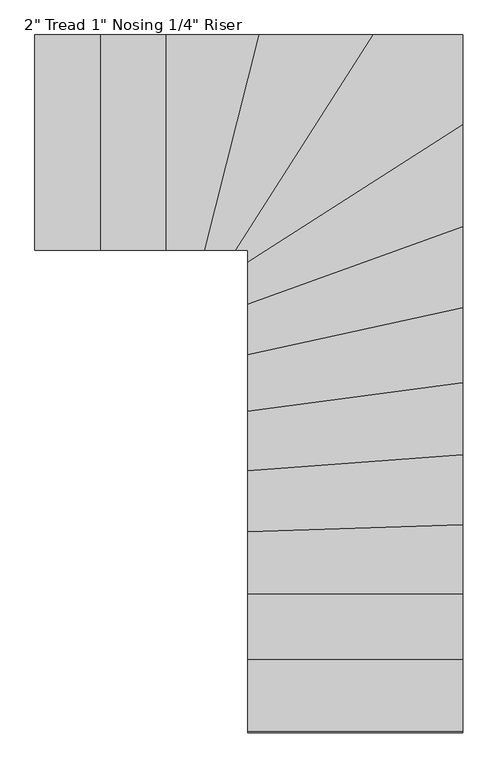
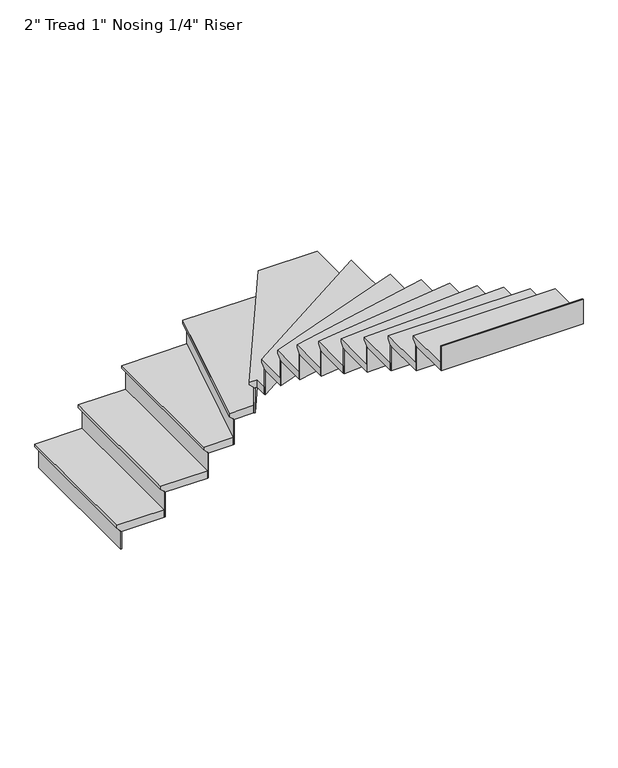
"""IFC4 building model written with IfcOpenShell, lengths in millimetres: stair flight geometry."""

from ifc_helpers import new_model, si_unit, origin, place, context, project, spatial, faceted_brep, source, transform, mapped, element, save


def stair_flight_29561c67(model_context):
    return source(origin(), model_context, "Body", "Brep", [
        faceted_brep([(-4406.7350785, 4803.7033005, 827.6166667), (-4406.7350785, 4803.7033005, 846.6666667), (-4406.7350785, 5718.1033005, 846.6666667), (-4406.7350785, 5718.1033005, 827.6166667), (-4381.3350785, 4803.7033005, 802.2166667), (-4381.3350785, 5718.1033005, 802.2166667), (-4101.9350785, 4803.7033005, 846.6666667), (-4101.9350785, 5718.1033005, 846.6666667), (-4381.3350785, 5718.1033005, 795.8666667), (-4101.9350785, 5718.1033005, 795.8666667), (-4101.9350785, 4803.7033005, 795.8666667), (-4381.3350785, 4803.7033005, 795.8666667)], [[[0, 1, 2, 3]], [[4, 0, 3, 5]], [[2, 1, 6, 7]], [[8, 9, 10, 11]], [[2, 7, 9, 8, 5, 3]], [[8, 11, 4, 5]], [[6, 1, 0, 4, 11, 10]], [[7, 6, 10, 9]]]),
        faceted_brep([(-4381.3350785, 4803.7033005, 795.8666667), (-4381.3350785, 4803.7033005, 677.3333333), (-4374.9850785, 4803.7033005, 677.3333333), (-4374.9850785, 4803.7033005, 795.8666667), (-4381.3350785, 5718.1033005, 795.8666667), (-4374.9850785, 5718.1033005, 795.8666667), (-4374.9850785, 5718.1033005, 677.3333333), (-4381.3350785, 5718.1033005, 677.3333333)], [[[0, 1, 2, 3]], [[4, 5, 6, 7]], [[1, 0, 4, 7]], [[2, 1, 7, 6]], [[3, 2, 6, 5]], [[0, 3, 5, 4]]]),
        faceted_brep([(-4101.9350785, 4803.7033005, 965.2), (-4101.9350785, 4803.7033005, 795.8666667), (-4095.5850785, 4803.7033005, 795.8666667), (-4095.5850785, 4803.7033005, 965.2), (-4101.9350785, 5718.1033005, 965.2), (-4095.5850785, 5718.1033005, 965.2), (-4095.5850785, 5718.1033005, 795.8666667), (-4101.9350785, 5718.1033005, 795.8666667)], [[[0, 1, 2, 3]], [[4, 5, 6, 7]], [[1, 0, 4, 7]], [[2, 1, 7, 6]], [[3, 2, 6, 5]], [[0, 3, 5, 4]]]),
        faceted_brep([(-4127.3350785, 5718.1033005, 1016.0), (-4127.3350785, 4803.7033005, 1016.0), (-3822.5350785, 4803.7033005, 1016.0), (-3822.5350785, 5718.1033005, 1016.0), (-4101.9350785, 5718.1033005, 965.2), (-3822.5350785, 5718.1033005, 965.2), (-3822.5350785, 4803.7033005, 965.2), (-4101.9350785, 4803.7033005, 965.2), (-4101.9350785, 5718.1033005, 971.55), (-4127.3350785, 5718.1033005, 996.95), (-4101.9350785, 4803.7033005, 971.55), (-4127.3350785, 4803.7033005, 996.95)], [[[0, 1, 2, 3]], [[4, 5, 6, 7]], [[0, 3, 5, 4, 8, 9]], [[4, 7, 10, 8]], [[2, 1, 11, 10, 7, 6]], [[3, 2, 6, 5]], [[11, 1, 0, 9]], [[10, 11, 9, 8]]]),
        faceted_brep([(-3822.5350785, 4803.7033005, 1134.5333333), (-3822.5350785, 4803.7033005, 965.2), (-3816.1850785, 4803.7033005, 965.2), (-3816.1850785, 4803.7033005, 1134.5333333), (-3822.5350785, 5718.1033005, 1134.5333333), (-3816.1850785, 5718.1033005, 1134.5333333), (-3816.1850785, 5718.1033005, 965.2), (-3822.5350785, 5718.1033005, 965.2)], [[[0, 1, 2, 3]], [[4, 5, 6, 7]], [[1, 0, 4, 7]], [[2, 1, 7, 6]], [[3, 2, 6, 5]], [[0, 3, 5, 4]]]),
        faceted_brep([(-3847.9350785, 5718.1033005, 1185.3333333), (-3847.9350785, 4803.7033005, 1185.3333333), (-3657.8300447, 4803.7033005, 1185.3333333), (-3426.8443681, 5718.1033005, 1185.3333333), (-3822.5350785, 5718.1033005, 1134.5333333), (-3426.8443681, 5718.1033005, 1134.5333333), (-3657.8300447, 4803.7033005, 1134.5333333), (-3822.5350785, 4803.7033005, 1134.5333333), (-3822.5350785, 5718.1033005, 1140.8833333), (-3847.9350785, 5718.1033005, 1166.2833333), (-3822.5350785, 4803.7033005, 1140.8833333), (-3847.9350785, 4803.7033005, 1166.2833333)], [[[0, 1, 2, 3]], [[4, 5, 6, 7]], [[0, 3, 5, 4, 8, 9]], [[4, 7, 10, 8]], [[2, 1, 11, 10, 7, 6]], [[3, 2, 6, 5]], [[11, 1, 0, 9]], [[10, 11, 9, 8]]]),
        faceted_brep([(-3657.8300447, 4803.7033005, 1303.8666667), (-3657.8300447, 4803.7033005, 1134.5333333), (-3651.2805766, 4803.7033005, 1134.5333333), (-3651.2805766, 4803.7033005, 1303.8666667), (-3426.8443681, 5718.1033005, 1303.8666667), (-3420.2949, 5718.1033005, 1303.8666667), (-3420.2949, 5718.1033005, 1134.5333333), (-3426.8443681, 5718.1033005, 1134.5333333)], [[[0, 1, 2, 3]], [[4, 5, 6, 7]], [[1, 0, 4, 7]], [[2, 1, 7, 6]], [[3, 2, 6, 5]], [[0, 3, 5, 4]]]),
        faceted_brep([(-3453.0422402, 5718.1033005, 1354.6666667), (-3684.0279168, 4803.7033005, 1354.6666667), (-3523.5624556, 4803.7033005, 1354.6666667), (-2938.9630202, 5718.1033005, 1354.6666667), (-3426.8443681, 5718.1033005, 1303.8666667), (-2938.9630202, 5718.1033005, 1303.8666667), (-3523.5624556, 4803.7033005, 1303.8666667), (-3657.8300447, 4803.7033005, 1303.8666667), (-3426.8443681, 5718.1033005, 1310.2166667), (-3453.0422402, 5718.1033005, 1335.6166667), (-3657.8300447, 4803.7033005, 1310.2166667), (-3684.0279168, 4803.7033005, 1335.6166667)], [[[0, 1, 2, 3]], [[4, 5, 6, 7]], [[0, 3, 5, 4, 8, 9]], [[4, 7, 10, 8]], [[2, 1, 11, 10, 7, 6]], [[3, 2, 6, 5]], [[11, 1, 0, 9]], [[10, 11, 9, 8]]]),
        faceted_brep([(-3523.5624556, 4803.7033005, 1473.2), (-3523.5624556, 4803.7033005, 1303.8666667), (-3516.0256252, 4803.7033005, 1303.8666667), (-3516.0256252, 4803.7033005, 1473.2), (-2938.9630202, 5718.1033005, 1473.2), (-2931.4261898, 5718.1033005, 1473.2), (-2931.4261898, 5718.1033005, 1303.8666667), (-2938.9630202, 5718.1033005, 1303.8666667)], [[[0, 1, 2, 3]], [[4, 5, 6, 7]], [[1, 0, 4, 7]], [[2, 1, 7, 6]], [[3, 2, 6, 5]], [[0, 3, 5, 4]]]),
        faceted_brep([(-2588.398089, 5307.243726, 1524.0), (-2588.398089, 5718.1033005, 1524.0), (-2969.1103419, 5718.1033005, 1524.0), (-3553.7097773, 4803.7033005, 1524.0), (-3502.798089, 4803.7033005, 1524.0), (-3502.798089, 4722.6442906, 1524.0), (-2588.398089, 5718.1033005, 1473.2), (-2588.398089, 5307.243726, 1473.2), (-3502.798089, 4722.6442906, 1473.2), (-3502.798089, 4803.7033005, 1473.2), (-3523.5624556, 4803.7033005, 1473.2), (-2938.9630202, 5718.1033005, 1473.2), (-3523.5624556, 4803.7033005, 1479.55), (-2938.9630202, 5718.1033005, 1479.55), (-3553.7097773, 4803.7033005, 1504.95), (-2969.1103419, 5718.1033005, 1504.95)], [[[0, 1, 2, 3, 4, 5]], [[6, 7, 8, 9, 10, 11]], [[1, 0, 7, 6]], [[11, 10, 12, 13]], [[4, 3, 14, 12, 10, 9]], [[0, 5, 8, 7]], [[14, 3, 2, 15]], [[12, 14, 15, 13]], [[2, 1, 6, 11, 13, 15]], [[5, 4, 9, 8]]]),
        faceted_brep([(-3502.798089, 4722.6442906, 1642.5333333), (-3502.798089, 4722.6442906, 1473.2), (-3502.798089, 4715.1074602, 1473.2), (-3502.798089, 4715.1074602, 1642.5333333), (-2588.398089, 5307.243726, 1642.5333333), (-2588.398089, 5299.7068956, 1642.5333333), (-2588.398089, 5299.7068956, 1473.2), (-2588.398089, 5307.243726, 1473.2)], [[[0, 1, 2, 3]], [[4, 5, 6, 7]], [[1, 0, 4, 7]], [[2, 1, 7, 6]], [[3, 2, 6, 5]], [[0, 3, 5, 4]]]),
        faceted_brep([(-2588.398089, 5337.3910477, 1693.3333333), (-3502.798089, 4752.7916123, 1693.3333333), (-3502.798089, 4546.6879787, 1693.3333333), (-2588.398089, 4875.2644835, 1693.3333333), (-2588.398089, 5307.243726, 1642.5333333), (-2588.398089, 4875.2644835, 1642.5333333), (-3502.798089, 4546.6879787, 1642.5333333), (-3502.798089, 4722.6442906, 1642.5333333), (-2588.398089, 5307.243726, 1648.8833333), (-2588.398089, 5337.3910477, 1674.2833333), (-3502.798089, 4722.6442906, 1648.8833333), (-3502.798089, 4752.7916123, 1674.2833333)], [[[0, 1, 2, 3]], [[4, 5, 6, 7]], [[0, 3, 5, 4, 8, 9]], [[4, 7, 10, 8]], [[2, 1, 11, 10, 7, 6]], [[3, 2, 6, 5]], [[11, 1, 0, 9]], [[10, 11, 9, 8]]]),
        faceted_brep([(-3502.798089, 4546.6879787, 1811.8666667), (-3502.798089, 4546.6879787, 1642.5333333), (-3502.798089, 4539.9404588, 1642.5333333), (-3502.798089, 4539.9404588, 1811.8666667), (-2588.398089, 4875.2644835, 1811.8666667), (-2588.398089, 4868.5169635, 1811.8666667), (-2588.398089, 4868.5169635, 1642.5333333), (-2588.398089, 4875.2644835, 1642.5333333)], [[[0, 1, 2, 3]], [[4, 5, 6, 7]], [[1, 0, 4, 7]], [[2, 1, 7, 6]], [[3, 2, 6, 5]], [[0, 3, 5, 4]]]),
        faceted_brep([(-2588.398089, 4902.2545634, 1862.6666667), (-3502.798089, 4573.6780586, 1862.6666667), (-3502.798089, 4332.5715797, 1862.6666667), (-2588.398089, 4532.5602463, 1862.6666667), (-2588.398089, 4875.2644835, 1811.8666667), (-2588.398089, 4532.5602463, 1811.8666667), (-3502.798089, 4332.5715797, 1811.8666667), (-3502.798089, 4546.6879787, 1811.8666667), (-2588.398089, 4875.2644835, 1818.2166667), (-2588.398089, 4902.2545634, 1843.6166667), (-3502.798089, 4546.6879787, 1818.2166667), (-3502.798089, 4573.6780586, 1843.6166667)], [[[0, 1, 2, 3]], [[4, 5, 6, 7]], [[0, 3, 5, 4, 8, 9]], [[4, 7, 10, 8]], [[2, 1, 11, 10, 7, 6]], [[3, 2, 6, 5]], [[11, 1, 0, 9]], [[10, 11, 9, 8]]]),
        faceted_brep([(-3502.798089, 4332.5715797, 1981.2), (-3502.798089, 4332.5715797, 1811.8666667), (-3502.798089, 4326.0714802, 1811.8666667), (-3502.798089, 4326.0714802, 1981.2), (-2588.398089, 4532.5602463, 1981.2), (-2588.398089, 4526.0601468, 1981.2), (-2588.398089, 4526.0601468, 1811.8666667), (-2588.398089, 4532.5602463, 1811.8666667)], [[[0, 1, 2, 3]], [[4, 5, 6, 7]], [[1, 0, 4, 7]], [[2, 1, 7, 6]], [[3, 2, 6, 5]], [[0, 3, 5, 4]]]),
        faceted_brep([(-2588.398089, 4558.5606443, 2032.0), (-3502.798089, 4358.5719777, 2032.0), (-3502.798089, 4093.0245396, 2032.0), (-2588.398089, 4214.0649516, 2032.0), (-2588.398089, 4532.5602463, 1981.2), (-2588.398089, 4214.0649516, 1981.2), (-3502.798089, 4093.0245396, 1981.2), (-3502.798089, 4332.5715797, 1981.2), (-2588.398089, 4532.5602463, 1987.55), (-2588.398089, 4558.5606443, 2012.95), (-3502.798089, 4332.5715797, 1987.55), (-3502.798089, 4358.5719777, 2012.95)], [[[0, 1, 2, 3]], [[4, 5, 6, 7]], [[0, 3, 5, 4, 8, 9]], [[4, 7, 10, 8]], [[2, 1, 11, 10, 7, 6]], [[3, 2, 6, 5]], [[11, 1, 0, 9]], [[10, 11, 9, 8]]]),
        faceted_brep([(-3502.798089, 4093.0245396, 2150.5333333), (-3502.798089, 4093.0245396, 1981.2), (-3502.798089, 4086.6191482, 1981.2), (-3502.798089, 4086.6191482, 2150.5333333), (-2588.398089, 4214.0649516, 2150.5333333), (-2588.398089, 4207.6595603, 2150.5333333), (-2588.398089, 4207.6595603, 1981.2), (-2588.398089, 4214.0649516, 1981.2)], [[[0, 1, 2, 3]], [[4, 5, 6, 7]], [[1, 0, 4, 7]], [[2, 1, 7, 6]], [[3, 2, 6, 5]], [[0, 3, 5, 4]]]),
        faceted_brep([(-2588.398089, 4239.6865171, 2201.3333333), (-3502.798089, 4118.646105, 2201.3333333), (-3502.798089, 3840.4778148, 2201.3333333), (-2588.398089, 3908.1160191, 2201.3333333), (-2588.398089, 4214.0649516, 2150.5333333), (-2588.398089, 3908.1160191, 2150.5333333), (-3502.798089, 3840.4778148, 2150.5333333), (-3502.798089, 4093.0245396, 2150.5333333), (-2588.398089, 4214.0649516, 2156.8833333), (-2588.398089, 4239.6865171, 2182.2833333), (-3502.798089, 4093.0245396, 2156.8833333), (-3502.798089, 4118.646105, 2182.2833333)], [[[0, 1, 2, 3]], [[4, 5, 6, 7]], [[0, 3, 5, 4, 8, 9]], [[4, 7, 10, 8]], [[2, 1, 11, 10, 7, 6]], [[3, 2, 6, 5]], [[11, 1, 0, 9]], [[10, 11, 9, 8]]]),
        faceted_brep([(-3502.798089, 3840.4778148, 2319.8666667), (-3502.798089, 3840.4778148, 2150.5333333), (-3502.798089, 3834.1104663, 2150.5333333), (-3502.798089, 3834.1104663, 2319.8666667), (-2588.398089, 3908.1160191, 2319.8666667), (-2588.398089, 3901.7486705, 2319.8666667), (-2588.398089, 3901.7486705, 2150.5333333), (-2588.398089, 3908.1160191, 2150.5333333)], [[[0, 1, 2, 3]], [[4, 5, 6, 7]], [[1, 0, 4, 7]], [[2, 1, 7, 6]], [[3, 2, 6, 5]], [[0, 3, 5, 4]]]),
        faceted_brep([(-2588.398089, 3933.5854132, 2370.6666667), (-3502.798089, 3865.9472089, 2370.6666667), (-3502.798089, 3580.3987016, 2370.6666667), (-2588.398089, 3609.5081857, 2370.6666667), (-2588.398089, 3908.1160191, 2319.8666667), (-2588.398089, 3609.5081857, 2319.8666667), (-3502.798089, 3580.3987016, 2319.8666667), (-3502.798089, 3840.4778148, 2319.8666667), (-2588.398089, 3908.1160191, 2326.2166667), (-2588.398089, 3933.5854132, 2351.6166667), (-3502.798089, 3840.4778148, 2326.2166667), (-3502.798089, 3865.9472089, 2351.6166667)], [[[0, 1, 2, 3]], [[4, 5, 6, 7]], [[0, 3, 5, 4, 8, 9]], [[4, 7, 10, 8]], [[2, 1, 11, 10, 7, 6]], [[3, 2, 6, 5]], [[11, 1, 0, 9]], [[10, 11, 9, 8]]]),
        faceted_brep([(-3502.798089, 3580.3987016, 2489.2), (-3502.798089, 3580.3987016, 2319.8666667), (-3502.798089, 3574.0454847, 2319.8666667), (-3502.798089, 3574.0454847, 2489.2), (-2588.398089, 3609.5081857, 2489.2), (-2588.398089, 3603.1549689, 2489.2), (-2588.398089, 3603.1549689, 2319.8666667), (-2588.398089, 3609.5081857, 2319.8666667)], [[[0, 1, 2, 3]], [[4, 5, 6, 7]], [[1, 0, 4, 7]], [[2, 1, 7, 6]], [[3, 2, 6, 5]], [[0, 3, 5, 4]]]),
        faceted_brep([(-2588.398089, 3634.9210531, 2540.0), (-3502.798089, 3605.811569, 2540.0), (-3502.798089, 3315.566311, 2540.0), (-2588.398089, 3315.566311, 2540.0), (-2588.398089, 3609.5081857, 2489.2), (-2588.398089, 3315.566311, 2489.2), (-3502.798089, 3315.566311, 2489.2), (-3502.798089, 3580.3987016, 2489.2), (-2588.398089, 3609.5081857, 2495.55), (-2588.398089, 3634.9210531, 2520.95), (-3502.798089, 3580.3987016, 2495.55), (-3502.798089, 3605.811569, 2520.95)], [[[0, 1, 2, 3]], [[4, 5, 6, 7]], [[0, 3, 5, 4, 8, 9]], [[4, 7, 10, 8]], [[2, 1, 11, 10, 7, 6]], [[3, 2, 6, 5]], [[11, 1, 0, 9]], [[10, 11, 9, 8]]]),
        faceted_brep([(-3502.798089, 3315.566311, 2658.5333333), (-3502.798089, 3315.566311, 2489.2), (-3502.798089, 3309.216311, 2489.2), (-3502.798089, 3309.216311, 2658.5333333), (-2588.398089, 3315.566311, 2658.5333333), (-2588.398089, 3309.216311, 2658.5333333), (-2588.398089, 3309.216311, 2489.2), (-2588.398089, 3315.566311, 2489.2)], [[[0, 1, 2, 3]], [[4, 5, 6, 7]], [[1, 0, 4, 7]], [[2, 1, 7, 6]], [[3, 2, 6, 5]], [[0, 3, 5, 4]]]),
        faceted_brep([(-2588.398089, 3340.966311, 2709.3333333), (-3502.798089, 3340.966311, 2709.3333333), (-3502.798089, 3036.166311, 2709.3333333), (-2588.398089, 3036.166311, 2709.3333333), (-2588.398089, 3315.566311, 2658.5333333), (-2588.398089, 3036.166311, 2658.5333333), (-3502.798089, 3036.166311, 2658.5333333), (-3502.798089, 3315.566311, 2658.5333333), (-2588.398089, 3315.566311, 2664.8833333), (-2588.398089, 3340.966311, 2690.2833333), (-3502.798089, 3315.566311, 2664.8833333), (-3502.798089, 3340.966311, 2690.2833333)], [[[0, 1, 2, 3]], [[4, 5, 6, 7]], [[0, 3, 5, 4, 8, 9]], [[4, 7, 10, 8]], [[2, 1, 11, 10, 7, 6]], [[3, 2, 6, 5]], [[11, 1, 0, 9]], [[10, 11, 9, 8]]]),
        faceted_brep([(-3502.798089, 3036.166311, 2827.8666667), (-3502.798089, 3036.166311, 2658.5333333), (-3502.798089, 3029.816311, 2658.5333333), (-3502.798089, 3029.816311, 2827.8666667), (-2588.398089, 3036.166311, 2827.8666667), (-2588.398089, 3029.816311, 2827.8666667), (-2588.398089, 3029.816311, 2658.5333333), (-2588.398089, 3036.166311, 2658.5333333)], [[[0, 1, 2, 3]], [[4, 5, 6, 7]], [[1, 0, 4, 7]], [[2, 1, 7, 6]], [[3, 2, 6, 5]], [[0, 3, 5, 4]]]),
        faceted_brep([(-3502.798089, 2756.766311, 2997.2), (-3502.798089, 2756.766311, 2827.8666667), (-3502.798089, 2750.416311, 2827.8666667), (-3502.798089, 2750.416311, 2997.2), (-2588.398089, 2756.766311, 2997.2), (-2588.398089, 2750.416311, 2997.2), (-2588.398089, 2750.416311, 2827.8666667), (-2588.398089, 2756.766311, 2827.8666667)], [[[0, 1, 2, 3]], [[4, 5, 6, 7]], [[1, 0, 4, 7]], [[2, 1, 7, 6]], [[3, 2, 6, 5]], [[0, 3, 5, 4]]]),
        faceted_brep([(-2588.398089, 3061.566311, 2878.6666667), (-3502.798089, 3061.566311, 2878.6666667), (-3502.798089, 2756.766311, 2878.6666667), (-2588.398089, 2756.766311, 2878.6666667), (-2588.398089, 3036.166311, 2827.8666667), (-2588.398089, 2756.766311, 2827.8666667), (-3502.798089, 2756.766311, 2827.8666667), (-3502.798089, 3036.166311, 2827.8666667), (-2588.398089, 3036.166311, 2834.2166667), (-2588.398089, 3061.566311, 2859.6166667), (-3502.798089, 3036.166311, 2834.2166667), (-3502.798089, 3061.566311, 2859.6166667)], [[[0, 1, 2, 3]], [[4, 5, 6, 7]], [[0, 3, 5, 4, 8, 9]], [[4, 7, 10, 8]], [[2, 1, 11, 10, 7, 6]], [[3, 2, 6, 5]], [[11, 1, 0, 9]], [[10, 11, 9, 8]]]),
    ])


if __name__ == "__main__":
    model = new_model("IFC4")
    model_context = context("Model", 3, world=origin())
    ifc_project = project(units=[si_unit("LENGTHUNIT", "METRE", prefix="MILLI")], contexts=[model_context])
    site = spatial("IfcSite", under=ifc_project)
    building = spatial("IfcBuilding", under=site)
    placement = place(None, origin())
    stair_flight_shape = stair_flight_29561c67(model_context)
    element("IfcStairFlight", 1, ObjectType="2\" Tread 1\" Nosing 1/4\" Riser", at=placement, inside=building, context=model_context, shape_type="MappedRepresentation", body=[
        mapped(stair_flight_shape, transform((0.0, 0.0, 0.0), x_axis=(1.0, 0.0, 0.0), y_axis=(0.0, 1.0, 0.0), z_axis=(0.0, 0.0, 1.0))),
    ])
    save(model, "model.ifc")
